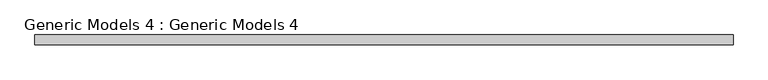
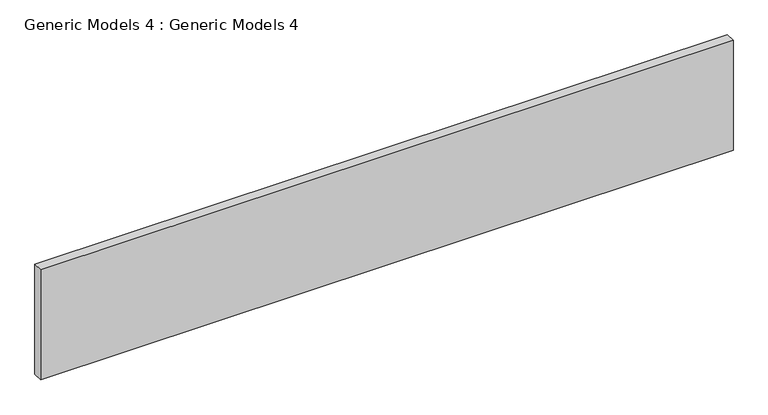
"""IFC4 building model written with IfcOpenShell, lengths in millimetres: proxy geometry, Generic Models 4 : Generic Models 4."""

from ifc_helpers import new_model, si_unit, frame, origin, place, context, project, spatial, polyline, outline, extrude, source, transform, mapped, element, save


def generic_models_4_generic_models_4_3414f660(model_context):
    return source(origin(), model_context, "Body", "SweptSolid", [
        extrude(outline(polyline([(497.6218735, -5887.8142532), (-3134.5781265, -5887.8142532), (-3134.5781265, -5837.0142532), (497.6218735, -5837.0142532), (497.6218735, -5887.8142532)])), frame((0.0, 0.0, 5791.2), z_axis=(0.0, 0.0, 1.0), x_axis=(1.0, 0.0, 0.0)), (0.0, 0.0, 1.0), 609.6),
    ])


if __name__ == "__main__":
    model = new_model("IFC4")
    model_context = context("Model", 3, world=origin())
    ifc_project = project(units=[si_unit("LENGTHUNIT", "METRE", prefix="MILLI")], contexts=[model_context])
    site = spatial("IfcSite", under=ifc_project)
    building = spatial("IfcBuilding", under=site)
    placement = place(None, origin())
    generic_models_4_generic_models_4_shape = generic_models_4_generic_models_4_3414f660(model_context)
    element("IfcBuildingElementProxy", 1, Name="Generic Models 4 : Generic Models 4", ObjectType="Generic Models 4 : Generic Models 4", at=placement, inside=building, context=model_context, shape_type="MappedRepresentation", body=[
        mapped(generic_models_4_generic_models_4_shape, transform((0.0, 0.0, 0.0), x_axis=(1.0, 0.0, 0.0), y_axis=(0.0, 1.0, 0.0), z_axis=(0.0, 0.0, 1.0))),
    ])
    save(model, "model.ifc")
